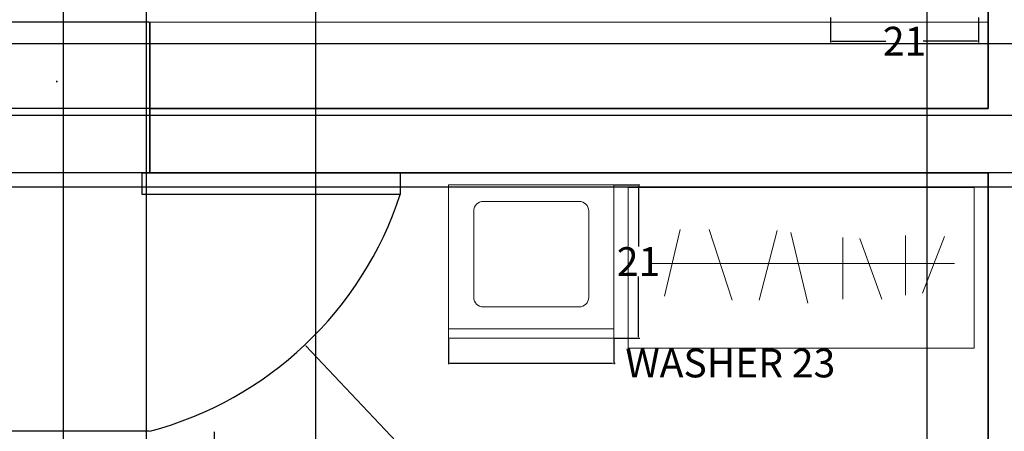
# Model space of a CAD drawing. Units: inches. Extents: x 1291 to 2095, y 532 to 1090.
# Tile 10 of 14: x 1559 to 1696, y 817 to 874. Entities that reach past the tile are written whole.
import ezdxf

# ---------------------------------------------------------------- set-up
doc = ezdxf.new("R2010")
doc.units = ezdxf.units.IN
doc.header["$MEASUREMENT"] = 0
for name, color, linetype, lineweight in [('A-ANNO-DIMS', 2, 'Continuous', 18), ('A-DOOR', 3, 'Continuous', 25), ('A-EQPM', 9, 'Continuous', 18), ('A-FLOR-CASE', 9, 'Continuous', 18), ('A-WALL', 7, 'Continuous', 35)]:
    doc.layers.add(name, color=color, linetype=linetype, lineweight=lineweight)
doc.styles.get("Standard").update_dxf_attribs({"font": 'arial.ttf'})
doc.dimstyles.get("Standard").update_dxf_attribs({"dimtxt": 4, "dimasz": 0.18, "dimexe": 0.18, "dimexo": 0.0625, "dimgap": 0.09, "dimtad": 0, "dimtih": 1, "dimtoh": 1, "dimdec": 0, "dimrnd": 6, "dimzin": 0, "dimdsep": 46, "dimlunit": 3, "dimtxsty": 'Standard', "dimcen": 0.09, "dimadec": 0, "dimazin": 0, "dimtfac": 1, "dimtdec": 0, "dimtofl": 0, "dimtmove": 0, "dimatfit": 3, "dimfxl": 1, "dimtolj": 1, "dimtzin": 0, "dimarcsym": 0})

# ---------------------------------------------------------------- blocks, each defined once
blk = doc.blocks.new('LAVADORA')
for p, q in [((-0.35, 0.65), (-0.35, 0)), ((-0.35, 0.65), (0.35, 0.65)), ((0.35, 0.65), (0.35, 0)), ((-0.2031, 0.5795), (0.2031, 0.5795)), ((-0.2437, 0.5389), (-0.2437, 0.1732)), ((0.2437, 0.5389), (0.2437, 0.1732)), ((-0.2031, 0.1326), (0.2031, 0.1326)), ((-0.35, 0.0406), (0.35, 0.0406)), ((-0.35, 0), (0.35, 0))]:
    blk.add_line(p, q)
for centre, start, end in [((-0.2031, 0.5389), 90, 180), ((0.2031, 0.5389), 0, 90), ((-0.2031, 0.1732), 180, 270), ((0.2031, 0.1732), 270, 0)]:
    blk.add_arc(centre, 0.0406, start, end)
blk = doc.blocks.new('*D17')
at = {"layer": 'A-ANNO-DIMS', "color": 0, "lineweight": -2, "transparency": 16777216}
for p, q in [((1672.08, 874.42), (1672.08, 870.96)), ((1692.74, 874.42), (1692.74, 870.96)), ((1672.26, 871.14), (1679.81, 871.14)), ((1692.56, 871.14), (1685.01, 871.14))]:
    blk.add_line(p, q, dxfattribs=at)
at = {"layer": 'A-ANNO-DIMS', "color": 0, "transparency": 16777216}
for points in [[(1672.26, 871.17), (1672.26, 871.11), (1672.08, 871.14)], [(1692.56, 871.17), (1692.56, 871.11), (1692.74, 871.14)]]:
    blk.add_solid(points, dxfattribs=at)
at = {"layer": 'Defpoints', "color": 0, "transparency": 16777216}
for p in [(1672.08, 874.48), (1692.74, 874.48), (1692.74, 871.14)]:
    blk.add_point(p, dxfattribs=at)
at = {"layer": 'A-ANNO-DIMS', "color": 0, "transparency": 16777216, "insert": (1682.41, 871.14), "char_height": 4, "attachment_point": 5}
blk.add_mtext('\\A1;21', dxfattribs=at)
blk = doc.blocks.new('*D18')
at = {"layer": 'A-ANNO-DIMS', "color": 0, "lineweight": -2, "transparency": 16777216}
for p, q in [((1618.79, 829.68), (1618.79, 826.11)), ((1641.83, 829.68), (1641.83, 826.11)), ((1618.97, 826.29), (1641.65, 826.29)), ((1641.83, 826.29), (1642.01, 826.29))]:
    blk.add_line(p, q, dxfattribs=at)
at = {"layer": 'A-ANNO-DIMS', "color": 0, "transparency": 16777216}
for points in [[(1618.97, 826.32), (1618.97, 826.26), (1618.79, 826.29)], [(1641.65, 826.32), (1641.65, 826.26), (1641.83, 826.29)]]:
    blk.add_solid(points, dxfattribs=at)
at = {"layer": 'Defpoints', "color": 0, "transparency": 16777216}
for p in [(1618.79, 829.74), (1641.83, 829.74), (1641.83, 826.29)]:
    blk.add_point(p, dxfattribs=at)
at = {"layer": 'A-ANNO-DIMS', "color": 0, "transparency": 16777216, "insert": (1658.09, 826.29), "char_height": 4, "attachment_point": 5}
blk.add_mtext('\\A1;WASHER 23', dxfattribs=at)
blk = doc.blocks.new('*D19')
at = {"layer": 'A-ANNO-DIMS', "color": 0, "lineweight": -2, "transparency": 16777216}
for p, q in [((1641.89, 851.13), (1645.46, 851.13)), ((1645.28, 850.95), (1645.28, 842.54)), ((1645.28, 829.92), (1645.28, 838.34)), ((1641.89, 829.74), (1645.46, 829.74))]:
    blk.add_line(p, q, dxfattribs=at)
at = {"layer": 'A-ANNO-DIMS', "color": 0, "transparency": 16777216}
for points in [[(1645.25, 850.95), (1645.31, 850.95), (1645.28, 851.13)], [(1645.25, 829.92), (1645.31, 829.92), (1645.28, 829.74)]]:
    blk.add_solid(points, dxfattribs=at)
at = {"layer": 'Defpoints', "color": 0, "transparency": 16777216}
for p in [(1641.83, 851.13), (1645.28, 851.13), (1641.83, 829.74)]:
    blk.add_point(p, dxfattribs=at)
at = {"layer": 'A-ANNO-DIMS', "color": 0, "transparency": 16777216, "insert": (1645.28, 840.44), "char_height": 4, "attachment_point": 5}
blk.add_mtext('\\A1;21', dxfattribs=at)
blk = doc.blocks.new('*D44')
at = {"layer": 'A-ANNO-DIMS', "color": 0, "lineweight": -2, "transparency": 16777216}
for p, q in [((1343.07, 579.84), (1343.07, 1087.16)), ((1343.25, 1086.98), (1451.42, 1086.98)), ((1576.43, 1086.98), (1468.26, 1086.98)), ((1576.61, 579.84), (1576.61, 1087.16))]:
    blk.add_line(p, q, dxfattribs=at)
at = {"layer": 'A-ANNO-DIMS', "color": 0, "transparency": 16777216}
for points in [[(1343.25, 1087.01), (1343.25, 1086.95), (1343.07, 1086.98)], [(1576.43, 1087.01), (1576.43, 1086.95), (1576.61, 1086.98)]]:
    blk.add_solid(points, dxfattribs=at)
at = {"layer": 'Defpoints', "color": 0, "transparency": 16777216}
for p in [(1576.61, 1086.98), (1343.07, 579.78), (1576.61, 579.78)]:
    blk.add_point(p, dxfattribs=at)
at = {"layer": 'A-ANNO-DIMS', "color": 0, "transparency": 16777216, "insert": (1459.84, 1086.98), "char_height": 4, "attachment_point": 5}
blk.add_mtext('\\A1;233.54', dxfattribs=at)
blk = doc.blocks.new('*D46')
at = {"layer": 'A-ANNO-DIMS', "color": 0, "lineweight": -2, "transparency": 16777216}
for p, q in [((1600.27, 579.84), (1600.27, 1087.16)), ((1600.45, 1086.98), (1636.47, 1086.98)), ((1685.4, 1086.98), (1649.38, 1086.98)), ((1685.58, 579.84), (1685.58, 1087.16))]:
    blk.add_line(p, q, dxfattribs=at)
at = {"layer": 'A-ANNO-DIMS', "color": 0, "transparency": 16777216}
for points in [[(1600.45, 1087.01), (1600.45, 1086.95), (1600.27, 1086.98)], [(1685.4, 1087.01), (1685.4, 1086.95), (1685.58, 1086.98)]]:
    blk.add_solid(points, dxfattribs=at)
at = {"layer": 'Defpoints', "color": 0, "transparency": 16777216}
for p in [(1685.58, 1086.98), (1600.27, 579.78), (1685.58, 579.78)]:
    blk.add_point(p, dxfattribs=at)
at = {"layer": 'A-ANNO-DIMS', "color": 0, "transparency": 16777216, "insert": (1642.93, 1086.98), "char_height": 4, "attachment_point": 5}
blk.add_mtext('\\A1;85.31', dxfattribs=at)
blk = doc.blocks.new('*D48')
at = {"layer": 'A-ANNO-DIMS', "color": 0, "lineweight": -2, "transparency": 16777216}
for p, q in [((1577.01, 852.78), (1297.69, 852.78)), ((1297.87, 852.6), (1297.87, 836.91)), ((1297.87, 816.96), (1297.87, 832.65)), ((1577.01, 816.78), (1297.69, 816.78))]:
    blk.add_line(p, q, dxfattribs=at)
at = {"layer": 'A-ANNO-DIMS', "color": 0, "transparency": 16777216}
for points in [[(1297.84, 852.6), (1297.9, 852.6), (1297.87, 852.78)], [(1297.84, 816.96), (1297.9, 816.96), (1297.87, 816.78)]]:
    blk.add_solid(points, dxfattribs=at)
at = {"layer": 'Defpoints', "color": 0, "transparency": 16777216}
for p in [(1297.87, 852.78), (1577.07, 852.78), (1577.07, 816.78)]:
    blk.add_point(p, dxfattribs=at)
at = {"layer": 'A-ANNO-DIMS', "color": 0, "transparency": 16777216, "insert": (1297.87, 834.78), "char_height": 4, "attachment_point": 5}
blk.add_mtext('\\A1;36', dxfattribs=at)
blk = doc.blocks.new('*D49')
at = {"layer": 'A-ANNO-DIMS', "color": 0, "lineweight": -2, "transparency": 16777216}
for p, q in [((1694.07, 852.72), (1694.07, 534.4)), ((1586.07, 816.72), (1586.07, 534.4)), ((1586.25, 534.58), (1635.75, 534.58)), ((1693.89, 534.58), (1644.4, 534.58))]:
    blk.add_line(p, q, dxfattribs=at)
at = {"layer": 'A-ANNO-DIMS', "color": 0, "transparency": 16777216}
for points in [[(1586.25, 534.61), (1586.25, 534.55), (1586.07, 534.58)], [(1693.89, 534.61), (1693.89, 534.55), (1694.07, 534.58)]]:
    blk.add_solid(points, dxfattribs=at)
at = {"layer": 'Defpoints', "color": 0, "transparency": 16777216}
for p in [(1694.07, 852.78), (1586.07, 816.78), (1694.07, 534.58)]:
    blk.add_point(p, dxfattribs=at)
at = {"layer": 'A-ANNO-DIMS', "color": 0, "transparency": 16777216, "insert": (1640.07, 534.58), "char_height": 4, "attachment_point": 5}
blk.add_mtext('\\A1;108', dxfattribs=at)
blk = doc.blocks.new('*D51')
at = {"layer": 'A-ANNO-DIMS', "color": 0, "lineweight": -2, "transparency": 16777216}
for p, q in [((1820.01, 852.78), (1297.69, 852.78)), ((1297.87, 852.6), (1297.87, 794.91)), ((1297.87, 732.96), (1297.87, 790.65)), ((1811.01, 732.78), (1297.69, 732.78))]:
    blk.add_line(p, q, dxfattribs=at)
at = {"layer": 'A-ANNO-DIMS', "color": 0, "transparency": 16777216}
for points in [[(1297.84, 852.6), (1297.9, 852.6), (1297.87, 852.78)], [(1297.84, 732.96), (1297.9, 732.96), (1297.87, 732.78)]]:
    blk.add_solid(points, dxfattribs=at)
at = {"layer": 'Defpoints', "color": 0, "transparency": 16777216}
for p in [(1297.87, 852.78), (1820.07, 852.78), (1811.07, 732.78)]:
    blk.add_point(p, dxfattribs=at)
at = {"layer": 'A-ANNO-DIMS', "color": 0, "transparency": 16777216, "insert": (1297.87, 792.78), "char_height": 4, "attachment_point": 5}
blk.add_mtext('\\A1;120', dxfattribs=at)
blk = doc.blocks.new('*D59')
at = {"layer": 'A-ANNO-DIMS', "color": 0, "lineweight": -2, "transparency": 16777216}
for p, q in [((2009.01, 900.78), (1297.69, 900.78)), ((1297.87, 900.6), (1297.87, 877.91)), ((1297.87, 850.96), (1297.87, 873.65)), ((2009.01, 850.78), (1297.69, 850.78))]:
    blk.add_line(p, q, dxfattribs=at)
at = {"layer": 'A-ANNO-DIMS', "color": 0, "transparency": 16777216}
for points in [[(1297.84, 900.6), (1297.9, 900.6), (1297.87, 900.78)], [(1297.84, 850.96), (1297.9, 850.96), (1297.87, 850.78)]]:
    blk.add_solid(points, dxfattribs=at)
at = {"layer": 'Defpoints', "color": 0, "transparency": 16777216}
for p in [(1297.87, 900.78), (2009.07, 900.78), (2009.07, 850.78)]:
    blk.add_point(p, dxfattribs=at)
at = {"layer": 'A-ANNO-DIMS', "color": 0, "transparency": 16777216, "insert": (1297.87, 875.78), "char_height": 4, "attachment_point": 5}
blk.add_mtext('\\A1;50', dxfattribs=at)
blk = doc.blocks.new('*D60')
at = {"layer": 'A-ANNO-DIMS', "color": 0, "lineweight": -2, "transparency": 16777216}
for p, q in [((2045.01, 870.78), (1297.69, 870.78)), ((1297.87, 870.6), (1297.87, 867.91)), ((1297.87, 860.96), (1297.87, 863.65)), ((2045.01, 860.78), (1297.69, 860.78))]:
    blk.add_line(p, q, dxfattribs=at)
at = {"layer": 'A-ANNO-DIMS', "color": 0, "transparency": 16777216}
for points in [[(1297.84, 870.6), (1297.9, 870.6), (1297.87, 870.78)], [(1297.84, 860.96), (1297.9, 860.96), (1297.87, 860.78)]]:
    blk.add_solid(points, dxfattribs=at)
at = {"layer": 'Defpoints', "color": 0, "transparency": 16777216}
for p in [(1297.87, 870.78), (2045.07, 870.78), (2045.07, 860.78)]:
    blk.add_point(p, dxfattribs=at)
at = {"layer": 'A-ANNO-DIMS', "color": 0, "transparency": 16777216, "insert": (1297.87, 865.78), "char_height": 4, "attachment_point": 5}
blk.add_mtext('\\A1;10', dxfattribs=at)
blk = doc.blocks.new('*D63')
at = {"layer": 'A-ANNO-DIMS', "color": 0, "lineweight": -2, "transparency": 16777216}
for p, q in [((1529.07, 723.84), (1529.07, 1087.16)), ((1529.25, 1086.98), (1544.12, 1086.98)), ((1564.89, 1086.98), (1550.03, 1086.98)), ((1565.07, 723.84), (1565.07, 1087.16))]:
    blk.add_line(p, q, dxfattribs=at)
at = {"layer": 'A-ANNO-DIMS', "color": 0, "transparency": 16777216}
for points in [[(1529.25, 1087.01), (1529.25, 1086.95), (1529.07, 1086.98)], [(1564.89, 1087.01), (1564.89, 1086.95), (1565.07, 1086.98)]]:
    blk.add_solid(points, dxfattribs=at)
at = {"layer": 'Defpoints', "color": 0, "transparency": 16777216}
for p in [(1565.07, 1086.98), (1529.07, 723.78), (1565.07, 723.78)]:
    blk.add_point(p, dxfattribs=at)
at = {"layer": 'A-ANNO-DIMS', "color": 0, "transparency": 16777216, "insert": (1547.07, 1086.98), "char_height": 4, "attachment_point": 5}
blk.add_mtext('\\A1;36', dxfattribs=at)
blk = doc.blocks.new('*D81')
at = {"layer": 'A-ANNO-DIMS', "color": 0, "lineweight": -2, "transparency": 16777216}
for p, q in [((1577.01, 873.78), (1297.69, 873.78)), ((1297.87, 873.6), (1297.87, 869.88)), ((1297.87, 861.96), (1297.87, 865.68)), ((1577.01, 861.78), (1297.69, 861.78))]:
    blk.add_line(p, q, dxfattribs=at)
at = {"layer": 'A-ANNO-DIMS', "color": 0, "transparency": 16777216}
for points in [[(1297.84, 873.6), (1297.9, 873.6), (1297.87, 873.78)], [(1297.84, 861.96), (1297.9, 861.96), (1297.87, 861.78)]]:
    blk.add_solid(points, dxfattribs=at)
at = {"layer": 'Defpoints', "color": 0, "transparency": 16777216}
for p in [(1297.87, 873.78), (1577.07, 873.78), (1577.07, 861.78)]:
    blk.add_point(p, dxfattribs=at)
at = {"layer": 'A-ANNO-DIMS', "color": 0, "transparency": 16777216, "insert": (1297.87, 867.78), "char_height": 4, "attachment_point": 5}
blk.add_mtext('\\A1;12', dxfattribs=at)
blk = doc.blocks.new('*D85')
at = {"layer": 'A-ANNO-DIMS', "color": 0, "lineweight": -2, "transparency": 16777216}
for p, q in [((1564.14, 865.42), (1564.14, 865.6)), ((1564.05, 865.51), (1564.23, 865.51)), ((1619.51, 806.84), (1598.87, 828.71)), ((1619.69, 806.84), (1619.51, 806.84))]:
    blk.add_line(p, q, dxfattribs=at)
at = {"layer": 'A-ANNO-DIMS', "color": 0, "transparency": 16777216}
blk.add_solid([(1598.89, 828.73), (1598.85, 828.69), (1598.74, 828.84)], dxfattribs=at)
at = {"layer": 'Defpoints', "color": 0, "transparency": 16777216}
for p in [(1564.14, 865.51), (1598.74, 828.84)]:
    blk.add_point(p, dxfattribs=at)
at = {"layer": 'A-ANNO-DIMS', "color": 0, "transparency": 16777216, "insert": (1628.42, 806.84), "char_height": 4, "attachment_point": 5}
blk.add_mtext('\\A1;R50.42', dxfattribs=at)

msp = doc.modelspace()

# ---------------------------------------------------------------- linework, layer by layer
at = {"layer": 'A-DOOR'}
msp.add_lwpolyline([(1612.0408, 852.7804), (1612.0408, 849.7804), (1576.0408, 849.7804), (1576.0408, 852.7804)], close=True, dxfattribs=at)
msp.add_arc((1564.1416, 865.5092), 50.4156, 284.862859, 341.821238, dxfattribs=at)
at = {"layer": 'A-FLOR-CASE'}
for p, q in [((1694.0735, 873.7804), (1577.0735, 873.7804)), ((1648.8922, 835.6019), (1651.118, 844.9148)), ((1655.1523, 844.9148), (1658.3519, 835.0459)), ((1662.1079, 835.0459), (1664.6119, 844.7758)), ((1666.5595, 844.4978), (1668.9244, 834.6289)), ((1673.7933, 835.1849), (1673.7933, 843.8028)), ((1676.1582, 843.6638), (1679.2187, 835.1849)), ((1682.5574, 835.7409), (1682.5574, 844.0808)), ((1684.9223, 836.0189), (1687.9828, 843.9418)), ((1646.9861, 840.1809), (1689.3786, 840.1809))]:
    msp.add_line(p, q, dxfattribs=at)
msp.add_lwpolyline([(1643.8204, 828.3537), (1692.1314, 828.3537), (1692.1314, 850.7704), (1643.8204, 850.7704)], close=True, dxfattribs=at)
at = {"layer": 'A-WALL'}
for p, q in [((1694.0735, 861.7804), (1694.0735, 936.7804)), ((1577.0735, 852.7804), (1577.0735, 873.7804)), ((1694.0735, 861.7804), (1577.0735, 861.7804)), ((1694.0735, 852.7804), (1577.0735, 852.7804)), ((1694.0735, 732.7804), (1694.0735, 852.7804))]:
    msp.add_line(p, q, dxfattribs=at)

# ---------------------------------------------------------------- block references
at = {"layer": 'A-EQPM', "xscale": 32.91238461506193, "yscale": 32.91238461506193, "zscale": 32.91238461506193}
msp.add_blockref('LAVADORA', (1630.3096, 829.741), dxfattribs=at)

# ---------------------------------------------------------------- dimensions: what is measured, and where the dimension line sits
at = {"layer": 'A-ANNO-DIMS'}
for base, p1, p2, override, picture, middle in [((1576.6107, 1086.9804), (1343.0735, 579.7804), (1576.6107, 579.7804), {"dimdec": 2, "dimlfac": 1, "dimrnd": 0, "dimzin": 0, "dimdsep": 46, "dimlunit": 2}, '*D44', (1459.8421, 1086.9804)), ((1565.0735, 1086.9804), (1529.0735, 723.7804), (1565.0735, 723.7804), {"dimdec": 0, "dimlfac": 1, "dimrnd": 0, "dimzin": 0, "dimdsep": 46, "dimlunit": 2}, '*D63', (1547.0735, 1086.9804)), ((1685.5842, 1086.9804), (1600.2697, 579.7804), (1685.5842, 579.7804), {"dimdec": 2, "dimlfac": 1, "dimrnd": 0, "dimzin": 0, "dimdsep": 46, "dimlunit": 2}, '*D46', (1642.927, 1086.9804)), ((1692.7372, 871.1441), (1672.0814, 874.4808), (1692.7372, 874.4808), {"dimdec": 0, "dimlfac": 1, "dimrnd": 0, "dimzin": 0, "dimdsep": 46, "dimlunit": 2}, '*D17', (1682.4093, 871.1441)), ((1694.0735, 534.5804), (1586.0735, 816.7804), (1694.0735, 852.7804), {"dimdec": 0, "dimlfac": 1, "dimrnd": 0, "dimzin": 0, "dimdsep": 46, "dimlunit": 2}, '*D49', (1640.0735, 534.5804))]:
    dim = msp.add_linear_dim(base=base, p1=p1, p2=p2, dimstyle='Standard', override=override, dxfattribs=at)
    dim.commit()
    dim.dimension.update_dxf_attribs({"geometry": picture, "text_midpoint": middle})
for base, p1, p2, picture, middle in [((1297.8735, 900.7804), (2009.0735, 850.7804), (2009.0735, 900.7804), '*D59', (1297.8735, 875.7804)), ((1297.8735, 873.7804), (1577.0735, 861.7804), (1577.0735, 873.7804), '*D81', (1297.8735, 867.7804)), ((1297.8735, 870.7804), (2045.0735, 860.7804), (2045.0735, 870.7804), '*D60', (1297.8735, 865.7804)), ((1297.8735, 852.7804), (1811.0735, 732.7804), (1820.0735, 852.7804), '*D51', (1297.8735, 792.7804)), ((1297.8735, 852.7804), (1577.0735, 816.7804), (1577.0735, 852.7804), '*D48', (1297.8735, 834.7804)), ((1645.2848, 851.134), (1641.829, 829.741), (1641.829, 851.134), '*D19', (1645.2848, 840.4375))]:
    dim = msp.add_linear_dim(base=base, p1=p1, p2=p2, angle=90, dimstyle='Standard', override={"dimdec": 0, "dimlfac": 1, "dimrnd": 0, "dimzin": 0, "dimdsep": 46, "dimlunit": 2}, dxfattribs=at)
    dim.commit()
    dim.dimension.update_dxf_attribs({"geometry": picture, "text_midpoint": middle})
dim = msp.add_radius_dim(center=(1564.1416, 865.5092), mpoint=(1598.7445, 828.8435), dimstyle='Standard', override={"dimdec": 2, "dimlfac": 1, "dimrnd": 0, "dimzin": 0, "dimdsep": 46, "dimlunit": 2}, dxfattribs=at)
dim.commit()
dim.dimension.update_dxf_attribs({"geometry": '*D85', "text_midpoint": (1628.4187, 806.8441), "dimtype": 164})
dim = msp.add_linear_dim(base=(1641.829, 826.2852), p1=(1618.7903, 829.741), p2=(1641.829, 829.741), text='WASHER <>', dimstyle='Standard', override={"dimdec": 0, "dimlfac": 1, "dimrnd": 0, "dimzin": 0, "dimdsep": 46, "dimlunit": 2}, dxfattribs=at)
dim.commit()
dim.dimension.update_dxf_attribs({"geometry": '*D18', "text_midpoint": (1658.0853, 826.2852)})

doc.saveas('drawing.dxf')
